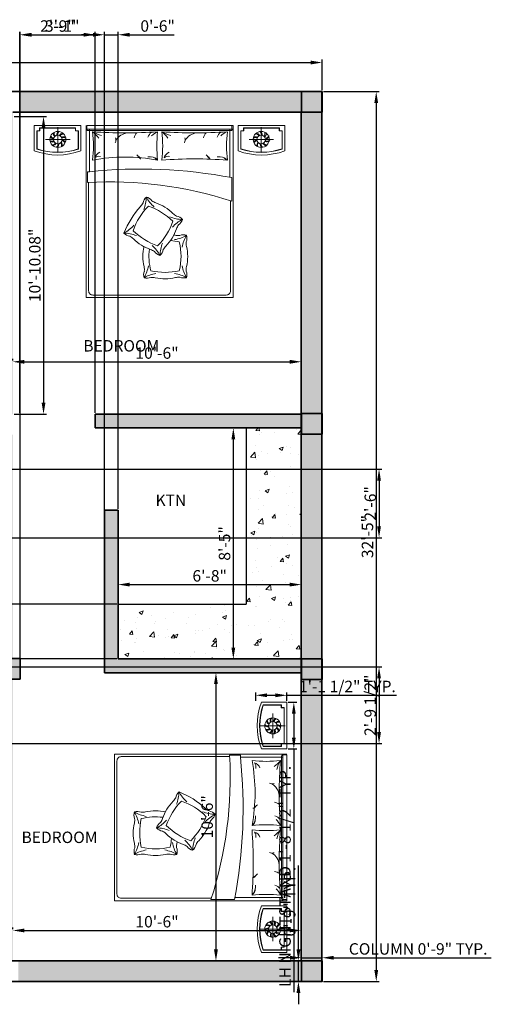
# Model space of a CAD drawing. Units: inches. Extents: x -36 to 490, y -420 to 94.
# Tile 4 of 4: x 284 to 490, y -385 to 45. Entities that reach past the tile are written whole.
import ezdxf

# ---------------------------------------------------------------- set-up
doc = ezdxf.new("R2010")
doc.units = ezdxf.units.IN
for name, color, linetype, lineweight in [('A-ANNO-DIMS', 2, 'Continuous', 18), ('A-AREA-IDEN', 1, 'Continuous', 18), ('A-COLS', 1, 'Continuous', 35), ('A-FLOR-FIXT', 8, 'Continuous', 25), ('A-FLOR-FIXT-PATT', 252, 'Continuous', 13), ('A-WALL', 7, 'Continuous', 35), ('furn', 8, 'Continuous', 18)]:
    doc.layers.add(name, color=color, linetype=linetype, lineweight=lineweight)
doc.layers.add('A-WALL-PATT', color=177, linetype='Continuous', lineweight=13, true_color=0x293189)
doc.styles.get("Standard").update_dxf_attribs({"font": 'arial.ttf'})
doc.dimstyles.new('ISO-25', dxfattribs={"dimtxt": 5, "dimasz": 5, "dimexe": 1.25, "dimexo": 0.625, "dimtad": 1, "dimlunit": 3, "dimtxsty": 'Standard', "dimcen": 2.5, "dimadec": 0, "dimazin": 0, "dimtfac": 1, "dimtmove": 0, "dimatfit": 3, "dimfxl": 1, "dimarcsym": 0})

# ---------------------------------------------------------------- blocks, each defined once
blk = doc.blocks.new('*D1')
at = {"layer": 'A-ANNO-DIMS', "color": 0, "lineweight": -2, "transparency": 16777216}
for p, q in [((280.98, -352.29), (280.98, -351.67)), ((285.98, -352.92), (401.98, -352.92)), ((406.98, -352.29), (406.98, -351.67))]:
    blk.add_line(p, q, dxfattribs=at)
at = {"layer": 'A-ANNO-DIMS', "color": 0, "transparency": 16777216}
for points in [[(285.98, -352.09), (285.98, -353.75), (280.98, -352.92)], [(401.98, -352.09), (401.98, -353.75), (406.98, -352.92)]]:
    blk.add_solid(points, dxfattribs=at)
at = {"layer": 'Defpoints', "color": 0, "transparency": 16777216}
for p in [(280.98, -352.92), (406.98, -352.92), (406.98, -352.92)]:
    blk.add_point(p, dxfattribs=at)
at = {"layer": 'A-ANNO-DIMS', "color": 0, "transparency": 16777216, "insert": (343.98, -349.74), "char_height": 5, "attachment_point": 5}
blk.add_mtext('10\'-6"', dxfattribs=at)
blk = doc.blocks.new('*D2')
at = {"layer": 'A-ANNO-DIMS', "color": 0, "lineweight": -2, "transparency": 16777216}
for p, q in [((347.38, -240.23), (370.97, -240.23)), ((369.72, -245.23), (369.72, -361.23)), ((347.38, -366.23), (370.97, -366.23))]:
    blk.add_line(p, q, dxfattribs=at)
at = {"layer": 'A-ANNO-DIMS', "color": 0, "transparency": 16777216}
for points in [[(368.88, -245.23), (370.55, -245.23), (369.72, -240.23)], [(368.88, -361.23), (370.55, -361.23), (369.72, -366.23)]]:
    blk.add_solid(points, dxfattribs=at)
at = {"layer": 'Defpoints', "color": 0, "transparency": 16777216}
for p in [(346.75, -240.23), (346.75, -366.23), (369.72, -366.23)]:
    blk.add_point(p, dxfattribs=at)
at = {"layer": 'A-ANNO-DIMS', "color": 0, "transparency": 16777216, "insert": (366.54, -303.23), "char_height": 5, "attachment_point": 5, "rotation": 90}
blk.add_mtext('10\'-6"', dxfattribs=at)
blk = doc.blocks.new('*D15')
at = {"layer": 'A-ANNO-DIMS', "color": 0, "lineweight": -2, "transparency": 16777216}
for p, q in [((281.61, 2.85), (295.66, 2.85)), ((294.41, -2.15), (294.41, -122.23)), ((281.61, -127.23), (295.66, -127.23))]:
    blk.add_line(p, q, dxfattribs=at)
at = {"layer": 'A-ANNO-DIMS', "color": 0, "transparency": 16777216}
for points in [[(293.58, -2.15), (295.25, -2.15), (294.41, 2.85)], [(293.58, -122.23), (295.25, -122.23), (294.41, -127.23)]]:
    blk.add_solid(points, dxfattribs=at)
at = {"layer": 'Defpoints', "color": 0, "transparency": 16777216}
for p in [(280.98, 2.85), (280.98, -127.23), (294.41, -127.23)]:
    blk.add_point(p, dxfattribs=at)
at = {"layer": 'A-ANNO-DIMS', "color": 0, "transparency": 16777216, "insert": (291.24, -62.19), "char_height": 5, "attachment_point": 5, "rotation": 90}
blk.add_mtext('10\'-10.08"', dxfattribs=at)
blk = doc.blocks.new('*D16')
at = {"layer": 'A-ANNO-DIMS', "color": 0, "lineweight": -2, "transparency": 16777216}
for p, q in [((280.98, -103.71), (280.98, -103.08)), ((406.98, -103.71), (406.98, -103.08)), ((285.98, -104.33), (401.98, -104.33))]:
    blk.add_line(p, q, dxfattribs=at)
at = {"layer": 'A-ANNO-DIMS', "color": 0, "transparency": 16777216}
for points in [[(285.98, -103.5), (285.98, -105.17), (280.98, -104.33)], [(401.98, -103.5), (401.98, -105.17), (406.98, -104.33)]]:
    blk.add_solid(points, dxfattribs=at)
at = {"layer": 'Defpoints', "color": 0, "transparency": 16777216}
for p in [(280.98, -104.33), (406.98, -104.33), (406.98, -104.33)]:
    blk.add_point(p, dxfattribs=at)
at = {"layer": 'A-ANNO-DIMS', "color": 0, "transparency": 16777216, "insert": (343.98, -101.16), "char_height": 5, "attachment_point": 5}
blk.add_mtext('10\'-6"', dxfattribs=at)
blk = doc.blocks.new('*D19')
at = {"layer": 'A-ANNO-DIMS', "color": 0, "lineweight": -2, "transparency": 16777216}
for p, q in [((326.98, -201.1), (326.98, -200.48)), ((331.98, -201.73), (401.98, -201.73)), ((406.98, -201.1), (406.98, -200.48))]:
    blk.add_line(p, q, dxfattribs=at)
at = {"layer": 'A-ANNO-DIMS', "color": 0, "transparency": 16777216}
for points in [[(331.98, -200.9), (331.98, -202.56), (326.98, -201.73)], [(401.98, -200.9), (401.98, -202.56), (406.98, -201.73)]]:
    blk.add_solid(points, dxfattribs=at)
at = {"layer": 'Defpoints', "color": 0, "transparency": 16777216}
for p in [(326.98, -201.73), (406.98, -201.73), (406.98, -201.73)]:
    blk.add_point(p, dxfattribs=at)
at = {"layer": 'A-ANNO-DIMS', "color": 0, "transparency": 16777216, "insert": (366.98, -198.55), "char_height": 5, "attachment_point": 5}
blk.add_mtext('6\'-8"', dxfattribs=at)
blk = doc.blocks.new('*D20')
at = {"layer": 'A-ANNO-DIMS', "color": 0, "lineweight": -2, "transparency": 16777216}
for p, q in [((366.67, -133.23), (378.56, -133.23)), ((377.31, -138.23), (377.31, -229.23)), ((366.67, -234.23), (378.56, -234.23))]:
    blk.add_line(p, q, dxfattribs=at)
at = {"layer": 'A-ANNO-DIMS', "color": 0, "transparency": 16777216}
for points in [[(376.48, -138.23), (378.14, -138.23), (377.31, -133.23)], [(376.48, -229.23), (378.14, -229.23), (377.31, -234.23)]]:
    blk.add_solid(points, dxfattribs=at)
at = {"layer": 'Defpoints', "color": 0, "transparency": 16777216}
for p in [(366.05, -133.23), (366.05, -234.23), (377.31, -234.23)]:
    blk.add_point(p, dxfattribs=at)
at = {"layer": 'A-ANNO-DIMS', "color": 0, "transparency": 16777216, "insert": (374.13, -183.73), "char_height": 5, "attachment_point": 5, "rotation": 90}
blk.add_mtext('8\'-5"', dxfattribs=at)
blk = doc.blocks.new('*D21')
at = {"layer": 'A-ANNO-DIMS', "color": 0, "lineweight": -2, "transparency": 16777216}
for p, q in [((-0.02, 14.4), (-0.02, 27.74)), ((4.98, 26.49), (411.1, 26.49)), ((416.1, 14.4), (416.1, 27.74))]:
    blk.add_line(p, q, dxfattribs=at)
at = {"layer": 'A-ANNO-DIMS', "color": 0, "transparency": 16777216}
for points in [[(4.98, 27.33), (4.98, 25.66), (-0.02, 26.49)], [(411.1, 27.33), (411.1, 25.66), (416.1, 26.49)]]:
    blk.add_solid(points, dxfattribs=at)
at = {"layer": 'Defpoints', "color": 0, "transparency": 16777216}
for p in [(416.1, 26.49), (-0.02, 13.77), (416.1, 13.77)]:
    blk.add_point(p, dxfattribs=at)
at = {"layer": 'A-ANNO-DIMS', "color": 0, "transparency": 16777216, "insert": (208.04, 29.67), "char_height": 5, "attachment_point": 5}
blk.add_mtext('34\'-8.11"', dxfattribs=at)
blk = doc.blocks.new('*D22')
at = {"layer": 'A-ANNO-DIMS', "color": 0, "lineweight": -2, "transparency": 16777216}
for p, q in [((416.72, 13.77), (440.97, 13.77)), ((439.72, 8.77), (439.72, -370.23)), ((416.72, -375.23), (440.97, -375.23))]:
    blk.add_line(p, q, dxfattribs=at)
at = {"layer": 'A-ANNO-DIMS', "color": 0, "transparency": 16777216}
for points in [[(438.89, 8.77), (440.55, 8.77), (439.72, 13.77)], [(438.89, -370.23), (440.55, -370.23), (439.72, -375.23)]]:
    blk.add_solid(points, dxfattribs=at)
at = {"layer": 'Defpoints', "color": 0, "transparency": 16777216}
for p in [(416.1, 13.77), (416.1, -375.23), (439.72, -375.23)]:
    blk.add_point(p, dxfattribs=at)
at = {"layer": 'A-ANNO-DIMS', "color": 0, "transparency": 16777216, "insert": (436.54, -180.73), "char_height": 5, "attachment_point": 5, "rotation": 90}
blk.add_mtext('32\'-5"', dxfattribs=at)
blk = doc.blocks.new('BED-DOUBLE')
for p, q in [((1.43, 73.57), (1.43, 55.04)), ((62.71, 73.57), (62.71, 52.63)), ((1.11, 73.01), (63.06, 73.01))]:
    blk.add_line(p, q)
for points in [[(0, 75.3), (0, 0), (64.18, 0), (64.18, 75.3)], [(63.58, 75.3), (63.58, 73.57), (0.37, 73.57), (0.37, 75.3), (64.18, 75.3)]]:
    blk.add_lwpolyline(points)
for points in [[(2.84, 60.1, 0.058596), (2.84, 72.5, 0.036889), (31.25, 72.5, 0.052163), (31.25, 60.1, 0.093111)], [(33.1, 60.1, 0.058596), (33.1, 72.5, 0.036648), (61.69, 72.5, 0.052163), (61.69, 60.1, 0.036967)], [(0.56, 55.04), (1.43, 55.04, -0.072944), (63.58, 52.45), (63.58, 42.16, 0.092568), (0.56, 50.32)]]:
    blk.add_lwpolyline(points, format="xyb", close=True)
for points in [[(1.11, 50.35), (1.11, 2.97, 0.414214), (2.97, 1.11), (61.21, 1.11, 0.414214), (63.06, 2.97), (63.06, 42.34)], [(25.2, 38.53, 0.091296), (26.33, 43.97, 0.091296), (29.75, 39.6, 0.091296)], [(20.61, 29.25, 0.111006), (31.2, 22.66, 0.119549), (37.88, 33.38, 0.107813), (27.32, 40)], [(27.26, 39.98, 0.121865), (20.61, 29.25, 0.121865)], [(36.64, 35.3, 0.091296), (42.07, 34.16, 0.091296), (37.69, 30.75, 0.091296)], [(21.95, 27.08, 0.091296), (16.52, 28.23, 0.091296), (20.9, 31.63, 0.091296)], [(32.26, 18.42, 0.159461), (33.7, 20.96, -0.076283), (34.84, 22.55, 0.115075), (39.49, 30.02, -0.076283), (40.42, 31.75, 0.159461), (42.07, 34.16)], [(38.64, 25.34, 0.091296), (43.86, 27.24, 0.091296), (41.94, 22.03, 0.091296)], [(43.86, 8.69, 0.159461), (43.73, 11.61, -0.076283), (43.86, 13.56, 0.115075), (43.86, 22.37, -0.076283), (43.73, 24.32, 0.159461), (43.86, 27.24)], [(28.24, 11.72, 0.111006), (40.71, 11.73, 0.119549), (40.71, 24.36, 0.033212), (36.88, 24.95)], [(33.39, 23.85, 0.091296), (32.26, 18.42, 0.091296), (28.84, 22.79)], [(30.52, 10.59, 0.091296), (25.31, 8.69, 0.091296), (27.23, 13.9, 0.091296)], [(41.94, 13.9, 0.091296), (43.86, 8.69, 0.091296), (38.64, 10.59)]]:
    blk.add_lwpolyline(points, format="xyb")
for centre, radius, start, end in [((1.11, 74.12), 1.11, 180, 270), ((63.06, 74.12), 1.11, 270, 0), ((9.44, 82.87), 12.28, 237.5379, 257.5233), ((-6.45, 60.91), 14.86, 36.4935, 51.2792), ((9.94, 68.98), 3.08, 335.8927, 16.1192), ((18.86, 65.15), 6.88, 96.6849, 148.3182), ((25.81, 69.06), 4.82, 141.8174, 169.8987), ((31.91, 68.38), 5.19, 130.5354, 160.3558), ((35.15, 64), 9.35, 114.6457, 134.1585), ((23.8, 60.91), 14.86, 36.4935, 51.2792), ((39.69, 82.87), 12.28, 237.5379, 257.5233), ((40.19, 68.98), 3.08, 335.8927, 16.1192), ((49.11, 65.15), 6.88, 96.6849, 148.3182), ((56.06, 69.06), 4.82, 141.8174, 169.8987), ((62.16, 68.38), 5.19, 130.5354, 160.3558), ((65.4, 64), 9.35, 114.6457, 134.1585), ((7.73, 59.82), 4.12, 114.2916, 160.9896), ((5.59, 58.96), 2.82, 76.4823, 128.5563), ((11.2, 51.48), 15.49, 36.2085, 45.0849), ((22.66, 60.63), 1.04, 353.7543, 77.2187), ((27.63, 56.56), 5.07, 44.406, 96.8342), ((28.58, 58.33), 3.21, 33.6349, 90.8456), ((37.98, 59.82), 4.12, 114.2916, 160.9896), ((35.84, 58.96), 2.82, 76.4823, 128.5563), ((41.46, 51.48), 15.49, 36.2085, 45.0849), ((52.91, 60.63), 1.04, 353.7543, 77.2187), ((57.88, 56.56), 5.07, 44.406, 96.8342), ((58.83, 58.33), 3.21, 33.6349, 90.8456), ((29.5, 40.5), 4.7, 132.4658, 168.7065), ((25.09, 39.6), 4.54, 37.2937, 74.0973), ((54.12, 12.85), 40.62, 138.3818, 157.7644), ((19.15, 44.34), 6.44, 315.5854, 333.0343), ((32.54, 47.52), 6.44, 233.2983, 250.7472), ((24.23, 23.07), 19.38, 45.1307, 71.3884), ((42.4, 41.42), 6.44, 225.7718, 243.2208), ((38.72, 31.4), 4.34, 39.4726, 79.6505), ((19.98, 31.41), 4.7, 222.6522, 258.8929), ((16.17, 21.05), 6.44, 45.7718, 63.2208), ((34.58, 8.4), 19.38, 77.0576, 78.7033), ((40.3, 33.58), 6.44, 257.6988, 275.1477), ((42.47, 23.13), 4.34, 71.3996, 111.5774), ((34.34, 39.4), 19.38, 225.1307, 251.3884), ((44.18, 17.97), 19.38, 166.8711, 193.1289), ((53.75, 18.1), 26.29, 173.1956, 194.0284), ((26.03, 14.95), 6.44, 53.2983, 70.7472), ((34.07, 23.48), 5.38, 218.7754, 250.3571), ((19.02, 12.17), 6.44, 355.0387, 12.4877), ((29.84, 9.96), 4.7, 159.3666, 195.6073), ((26.56, 13.23), 4.7, 254.5791, 290.8198), ((28.81, 2.42), 6.44, 77.6988, 95.1477), ((34.52, 27.6), 19.38, 257.0576, 283.3153), ((40.4, 2.45), 6.44, 85.2252, 102.6741), ((42.71, 13.95), 5.38, 250.7023, 282.284)]:
    blk.add_arc(centre, radius, start, end)
blk = doc.blocks.new('NIGHTSTAND-LAMP-L')
for p, q in [((10.31, 1.49), (10.31, 12.19)), ((4.96, 6.84), (15.66, 6.84))]:
    blk.add_line(p, q)
blk.add_lwpolyline([(0, 1.86), (0, 12.98), (20.4, 12.98), (20.4, 1.86, -0.181818)], format="xyb", close=True)
for points in [[(2.34, 11.87), (2.34, 10.65), (1.11, 10.65)], [(2.45, 11.87), (2.45, 10.54), (1.11, 10.54)], [(2.34, 11.87), (18.07, 11.87)], [(2.34, 11.76), (18.07, 11.76)], [(17.95, 11.87), (17.95, 10.54), (19.29, 10.54)], [(18.07, 11.87), (18.07, 10.65), (19.29, 10.65)]]:
    blk.add_lwpolyline(points)
for points in [[(19.29, 10.65), (19.29, 2.63, -0.167087), (1.11, 2.63), (1.11, 10.65)], [(19.18, 10.65), (19.18, 2.71, -0.165559), (1.22, 2.71), (1.22, 10.65)]]:
    blk.add_lwpolyline(points, format="xyb")
for radius in [3.49, 1.89]:
    blk.add_circle((10.31, 6.84), radius)
for centre, radius, start, end in [((10.62, 9.46), 2.24, 172.17, 218.4897), ((10.4, 9.41), 1.71, 160.3002, 220.538), ((12.1, 8.78), 2.24, 136.17, 182.4897), ((11.89, 8.87), 1.71, 124.3002, 184.538), ((12.89, 7.36), 2.24, 100.17, 146.4897), ((12.78, 7.55), 1.71, 88.3002, 148.538), ((7.89, 7.72), 1.71, 232.3002, 292.538), ((7.91, 7.94), 2.24, 244.17, 290.4897), ((9.02, 9.14), 2.24, 208.17, 254.4897), ((8.87, 8.97), 1.71, 196.3002, 256.538), ((7.84, 6.13), 1.71, 268.3002, 328.538), ((7.72, 6.33), 2.24, 280.17, 326.4897), ((8.72, 4.82), 1.71, 304.3002, 4.538), ((8.52, 4.9), 2.24, 316.17, 2.4897), ((10.22, 4.27), 1.71, 340.3002, 40.538), ((10, 4.22), 2.24, 352.17, 38.4897), ((12.7, 5.74), 2.24, 64.17, 110.4897), ((12.72, 5.96), 1.71, 52.3002, 112.538), ((11.74, 4.71), 1.71, 16.3002, 76.538), ((11.59, 4.54), 2.24, 28.17, 74.4897)]:
    blk.add_arc(centre, radius, start, end)
blk = doc.blocks.new('NIGHTSTAND-LAMP-R')
for p, q in [((10.1, 1.49), (10.1, 12.18)), ((15.45, 6.83), (4.75, 6.83))]:
    blk.add_line(p, q)
blk.add_lwpolyline([(20.4, 1.85), (20.4, 12.98), (0, 12.98), (0, 1.85, 0.181818)], format="xyb", close=True)
for points in [[(2.34, 11.87), (2.34, 10.65), (1.11, 10.65)], [(2.45, 11.87), (2.45, 10.53), (1.11, 10.53)], [(18.07, 11.87), (2.34, 11.87)], [(18.07, 11.76), (2.34, 11.76)], [(17.95, 11.87), (17.95, 10.53), (19.29, 10.53)], [(18.07, 11.87), (18.07, 10.65), (19.29, 10.65)]]:
    blk.add_lwpolyline(points)
for points in [[(1.11, 10.65), (1.11, 2.63, 0.167087), (19.29, 2.63), (19.29, 10.65)], [(1.22, 10.65), (1.22, 2.71, 0.165559), (19.18, 2.71), (19.18, 10.65)]]:
    blk.add_lwpolyline(points, format="xyb")
for radius in [3.49, 1.89]:
    blk.add_circle((10.1, 6.83), radius)
for centre, radius, start, end in [((7.62, 7.54), 1.71, 31.462, 91.6998), ((7.51, 7.35), 2.24, 33.5103, 79.83), ((8.51, 8.86), 1.71, 355.462, 55.6998), ((8.31, 8.77), 2.24, 357.5103, 43.83), ((10.01, 9.4), 1.71, 319.462, 19.6998), ((10.04, 9.55), 2.24, 321.5103, 7.83), ((7.68, 5.95), 1.71, 67.462, 127.6998), ((7.7, 5.73), 2.24, 69.5103, 115.83), ((8.81, 4.54), 2.24, 105.5103, 151.83), ((8.66, 4.7), 1.71, 103.462, 163.6998), ((10.41, 4.22), 2.24, 141.5103, 187.83), ((10.19, 4.27), 1.71, 139.462, 199.6998), ((11.88, 4.9), 2.24, 177.5103, 223.83), ((11.68, 4.81), 1.71, 175.462, 235.6998), ((12.68, 6.32), 2.24, 213.5103, 259.83), ((12.57, 6.13), 1.71, 211.462, 271.6998), ((12.74, 8.03), 2.24, 249.5103, 295.83), ((12.77, 7.81), 1.71, 247.462, 307.6998), ((11.79, 9.06), 1.71, 283.462, 343.6998), ((11.64, 9.23), 2.24, 285.5103, 331.83)]:
    blk.add_arc(centre, radius, start, end)
blk = doc.blocks.new('COLUMN-9X9')
h = blk.add_hatch(color=256)
h.dxf.hatch_style = 1
h.paths.add_polyline_path([(9, 0), (9, 9), (0, 9), (0, 0)])
blk.add_lwpolyline([(0, 9), (9, 9), (9, 0), (0, 0)], close=True)
blk = doc.blocks.new('*D28')
at = {"layer": 'A-ANNO-DIMS', "color": 0, "lineweight": -2, "transparency": 16777216}
for p, q in [((402.09, -364.85), (397.09, -364.85)), ((407.09, -365.57), (407.09, -363.6)), ((407.09, -364.85), (416.09, -364.85)), ((416.09, -365.57), (416.09, -363.6)), ((421.09, -364.85), (489.97, -364.85))]:
    blk.add_line(p, q, dxfattribs=at)
at = {"layer": 'A-ANNO-DIMS', "color": 0, "transparency": 16777216}
for points in [[(402.09, -364.01), (402.09, -365.68), (407.09, -364.85)], [(421.09, -364.01), (421.09, -365.68), (416.09, -364.85)]]:
    blk.add_solid(points, dxfattribs=at)
at = {"layer": 'Defpoints', "color": 0, "transparency": 16777216}
for p in [(416.09, -364.85), (407.09, -366.2), (416.09, -366.2)]:
    blk.add_point(p, dxfattribs=at)
at = {"layer": 'A-ANNO-DIMS', "color": 0, "transparency": 16777216, "insert": (458.03, -361.63), "char_height": 5, "attachment_point": 5}
blk.add_mtext('COLUMN 0\'-9" TYP.', dxfattribs=at)
blk = doc.blocks.new('*D29')
at = {"layer": 'A-ANNO-DIMS', "color": 0, "lineweight": -2, "transparency": 16777216}
for p, q in [((405.74, -361.2), (405.74, -324.47)), ((406.47, -366.2), (404.49, -366.2)), ((405.74, -375.2), (405.74, -366.2)), ((406.47, -375.2), (404.49, -375.2)), ((405.74, -380.2), (405.74, -385.2))]:
    blk.add_line(p, q, dxfattribs=at)
at = {"layer": 'A-ANNO-DIMS', "color": 0, "transparency": 16777216}
for points in [[(404.91, -361.2), (406.58, -361.2), (405.74, -366.2)], [(404.91, -380.2), (406.58, -380.2), (405.74, -375.2)]]:
    blk.add_solid(points, dxfattribs=at)
at = {"layer": 'Defpoints', "color": 0, "transparency": 16777216}
for p in [(405.74, -366.2), (407.09, -366.2), (407.09, -375.2)]:
    blk.add_point(p, dxfattribs=at)
at = {"layer": 'A-ANNO-DIMS', "color": 0, "transparency": 16777216, "insert": (402.57, -340.33), "char_height": 5, "attachment_point": 5, "rotation": 90}
blk.add_mtext('0\'-9" TYP.', dxfattribs=at)
blk = doc.blocks.new('*D32')
at = {"layer": 'A-ANNO-DIMS', "color": 0, "lineweight": -2, "transparency": 16777216}
for p, q in [((401.3, -253.17), (404.99, -253.17)), ((403.74, -258.17), (403.74, -268.58)), ((401.3, -273.58), (404.99, -273.58)), ((403.74, -273.58), (403.74, -379.94))]:
    blk.add_line(p, q, dxfattribs=at)
at = {"layer": 'A-ANNO-DIMS', "color": 0, "transparency": 16777216}
for points in [[(402.9, -258.17), (404.57, -258.17), (403.74, -253.17)], [(402.9, -268.58), (404.57, -268.58), (403.74, -273.58)]]:
    blk.add_solid(points, dxfattribs=at)
at = {"layer": 'Defpoints', "color": 0, "transparency": 16777216}
for p in [(400.68, -253.17), (400.68, -273.58), (403.74, -273.58)]:
    blk.add_point(p, dxfattribs=at)
at = {"layer": 'A-ANNO-DIMS', "color": 0, "transparency": 16777216, "insert": (400.53, -329.26), "char_height": 5, "attachment_point": 5, "rotation": 90}
blk.add_mtext('LH NIGHTSTAND 1\'-8 1/2" TYP.', dxfattribs=at)
blk = doc.blocks.new('*D33')
at = {"layer": 'A-ANNO-DIMS', "color": 0, "lineweight": -2, "transparency": 16777216}
for p, q in [((387.08, -252.55), (387.08, -248.86)), ((400.68, -252.55), (400.68, -248.86)), ((392.08, -250.11), (395.68, -250.11)), ((400.68, -250.11), (448.59, -250.11))]:
    blk.add_line(p, q, dxfattribs=at)
at = {"layer": 'A-ANNO-DIMS', "color": 0, "transparency": 16777216}
for points in [[(392.08, -249.28), (392.08, -250.95), (387.08, -250.11)], [(395.68, -249.28), (395.68, -250.95), (400.68, -250.11)]]:
    blk.add_solid(points, dxfattribs=at)
at = {"layer": 'Defpoints', "color": 0, "transparency": 16777216}
for p in [(387.08, -253.17), (400.68, -250.11), (400.68, -253.17)]:
    blk.add_point(p, dxfattribs=at)
at = {"layer": 'A-ANNO-DIMS', "color": 0, "transparency": 16777216, "insert": (427.13, -246.9), "char_height": 5, "attachment_point": 5}
blk.add_mtext('1\'-1 1/2" TYP.', dxfattribs=at)
blk = doc.blocks.new('*D41')
at = {"layer": 'A-ANNO-DIMS', "color": 0, "lineweight": -2, "transparency": 16777216}
for p, q in [((326.36, -210.23), (-26.2, -210.23)), ((-24.95, -215.23), (-24.95, -229.23)), ((326.36, -234.23), (-26.2, -234.23))]:
    blk.add_line(p, q, dxfattribs=at)
at = {"layer": 'A-ANNO-DIMS', "color": 0, "transparency": 16777216}
for points in [[(-25.78, -215.23), (-24.12, -215.23), (-24.95, -210.23)], [(-25.78, -229.23), (-24.12, -229.23), (-24.95, -234.23)]]:
    blk.add_solid(points, dxfattribs=at)
at = {"layer": 'Defpoints', "color": 0, "transparency": 16777216}
for p in [(326.98, -210.23), (-24.95, -234.23), (326.98, -234.23)]:
    blk.add_point(p, dxfattribs=at)
at = {"layer": 'A-ANNO-DIMS', "color": 0, "transparency": 16777216, "insert": (-28.13, -222.23), "char_height": 5, "attachment_point": 5, "rotation": 90}
blk.add_mtext('2\'-0"', dxfattribs=at)
blk = doc.blocks.new('*D44')
at = {"layer": 'A-ANNO-DIMS', "color": 0, "lineweight": -2, "transparency": 16777216}
for p, q in [((284.01, -126.62), (284.01, 39.87)), ((316.98, -126.6), (316.98, 39.87)), ((289.01, 38.62), (311.98, 38.62))]:
    blk.add_line(p, q, dxfattribs=at)
at = {"layer": 'A-ANNO-DIMS', "color": 0, "transparency": 16777216}
for points in [[(289.01, 39.45), (289.01, 37.79), (284.01, 38.62)], [(311.98, 39.45), (311.98, 37.79), (316.98, 38.62)]]:
    blk.add_solid(points, dxfattribs=at)
at = {"layer": 'Defpoints', "color": 0, "transparency": 16777216}
for p in [(316.98, 38.62), (284.01, -127.24), (316.98, -127.23)]:
    blk.add_point(p, dxfattribs=at)
at = {"layer": 'A-ANNO-DIMS', "color": 0, "transparency": 16777216, "insert": (300.5, 41.8), "char_height": 5, "attachment_point": 5}
blk.add_mtext('2\'-9"', dxfattribs=at)
blk = doc.blocks.new('*D45')
at = {"layer": 'A-ANNO-DIMS', "color": 0, "lineweight": -2, "transparency": 16777216}
for p, q in [((95.61, -151.23), (442.2, -151.23)), ((440.95, -156.23), (440.95, -176.23)), ((101.61, -181.23), (442.2, -181.23))]:
    blk.add_line(p, q, dxfattribs=at)
at = {"layer": 'A-ANNO-DIMS', "color": 0, "transparency": 16777216}
for points in [[(440.11, -156.23), (441.78, -156.23), (440.95, -151.23)], [(440.11, -176.23), (441.78, -176.23), (440.95, -181.23)]]:
    blk.add_solid(points, dxfattribs=at)
at = {"layer": 'Defpoints', "color": 0, "transparency": 16777216}
for p in [(94.98, -151.23), (100.98, -181.23), (440.95, -181.23)]:
    blk.add_point(p, dxfattribs=at)
at = {"layer": 'A-ANNO-DIMS', "color": 0, "transparency": 16777216, "insert": (437.77, -166.23), "char_height": 5, "attachment_point": 5, "rotation": 90}
blk.add_mtext('2\'-6"', dxfattribs=at)
blk = doc.blocks.new('*D47')
at = {"layer": 'A-ANNO-DIMS', "color": 0, "lineweight": -2, "transparency": 16777216}
for p, q in [((144.42, -237.73), (442.2, -237.73)), ((440.95, -242.73), (440.95, -266.23)), ((141.61, -271.23), (442.2, -271.23))]:
    blk.add_line(p, q, dxfattribs=at)
at = {"layer": 'A-ANNO-DIMS', "color": 0, "transparency": 16777216}
for points in [[(440.11, -242.73), (441.78, -242.73), (440.95, -237.73)], [(440.11, -266.23), (441.78, -266.23), (440.95, -271.23)]]:
    blk.add_solid(points, dxfattribs=at)
at = {"layer": 'Defpoints', "color": 0, "transparency": 16777216}
for p in [(143.79, -237.73), (140.98, -271.23), (440.95, -271.23)]:
    blk.add_point(p, dxfattribs=at)
at = {"layer": 'A-ANNO-DIMS', "color": 0, "transparency": 16777216, "insert": (437.74, -254.48), "char_height": 5, "attachment_point": 5, "rotation": 90}
blk.add_mtext('2\'-9 1/2"', dxfattribs=at)
blk = doc.blocks.new('*D48')
at = {"layer": 'A-ANNO-DIMS', "color": 0, "lineweight": -2, "transparency": 16777216}
for p, q in [((284.18, -242.43), (284.18, 39.87)), ((320.98, -239.6), (320.98, 39.87)), ((289.18, 38.62), (315.98, 38.62))]:
    blk.add_line(p, q, dxfattribs=at)
at = {"layer": 'A-ANNO-DIMS', "color": 0, "transparency": 16777216}
for points in [[(289.18, 39.45), (289.18, 37.79), (284.18, 38.62)], [(315.98, 39.45), (315.98, 37.79), (320.98, 38.62)]]:
    blk.add_solid(points, dxfattribs=at)
at = {"layer": 'Defpoints', "color": 0, "transparency": 16777216}
for p in [(320.98, 38.62), (320.98, -240.23), (284.18, -243.05)]:
    blk.add_point(p, dxfattribs=at)
at = {"layer": 'A-ANNO-DIMS', "color": 0, "transparency": 16777216, "insert": (302.58, 41.8), "char_height": 5, "attachment_point": 5}
blk.add_mtext('3\'-1"', dxfattribs=at)
blk = doc.blocks.new('*D49')
at = {"layer": 'A-ANNO-DIMS', "color": 0, "lineweight": -2, "transparency": 16777216}
for p, q in [((320.98, -168.6), (320.98, 39.87)), ((326.98, -168.6), (326.98, 39.87)), ((315.98, 38.62), (310.98, 38.62)), ((320.98, 38.62), (326.98, 38.62)), ((331.98, 38.62), (351.53, 38.62))]:
    blk.add_line(p, q, dxfattribs=at)
at = {"layer": 'A-ANNO-DIMS', "color": 0, "transparency": 16777216}
for points in [[(315.98, 39.45), (315.98, 37.79), (320.98, 38.62)], [(331.98, 39.45), (331.98, 37.79), (326.98, 38.62)]]:
    blk.add_solid(points, dxfattribs=at)
at = {"layer": 'Defpoints', "color": 0, "transparency": 16777216}
for p in [(326.98, 38.62), (320.98, -169.23), (326.98, -169.23)]:
    blk.add_point(p, dxfattribs=at)
at = {"layer": 'A-ANNO-DIMS', "color": 0, "transparency": 16777216, "insert": (344.25, 41.8), "char_height": 5, "attachment_point": 5}
blk.add_mtext('0\'-6"', dxfattribs=at)

msp = doc.modelspace()

# ---------------------------------------------------------------- hatches: boundary and pattern name
at = {"layer": 'A-FLOR-FIXT-PATT'}
h = msp.add_hatch(dxfattribs=at)
h.set_pattern_fill('AR-CONC', color=256, scale=0.1)
h.set_pattern_definition([(50, (-137.025, -13.273), (18.21847, -1.5939), [1.905, -20.955]), (355, (-137.025, -13.273), (-3.52434, 19.1057), [1.524, -16.76406]), (100.4514, (-135.507, -13.406), (14.6941, 17.5118), [1.619, -17.809]), (46.184, (-137.025, -8.193), (27.1079, -4.2042), [2.8575, -31.4325]), (96.6356, (-134.766, -8.544), (23.7404, 24.7426), [2.4285, -26.7136]), (351.184, (-137.025, -8.193), (23.7404, 24.7426), [2.286, -25.146]), (21, (-134.485, -9.463), (15.16144, -10.22652), [1.905, -20.955]), (326, (-134.485, -9.463), (6.1802, 18.4188), [1.524, -16.764]), (71.4514, (-133.222, -10.316), (21.34164, 8.1923), [1.619, -17.809]), (37.5, (-137.025, -13.2735), (0.30886, 8.455504), [0, -16.5608, 0, -17.018, 0, -16.8275]), (7.5, (-137.025, -13.2735), (6.68197, 10.01806), [0, -9.7028, 0, -16.1798, 0, -6.4135]), (327.5, (-142.6895, -13.2735), (13.55906, -0.572874), [0, -6.35, 0, -19.812, 0, -26.289]), (317.5, (-145.23, -13.273), (14.81292, 2.54265), [0, -8.255, 0, -13.1572, 0, -18.669])])
h.paths.add_polyline_path([(406.984, -133.228), (382.984, -133.228), (382.984, -210.228), (326.984, -210.228), (326.984, -234.228), (406.984, -234.228)])
at = {"layer": 'A-WALL-PATT'}
h = msp.add_hatch(color=256, dxfattribs=at)
h.dxf.hatch_style = 1
h.paths.add_polyline_path([(132.114, 13.772), (8.901, 13.772), (8.901, 4.772), (132.114, 4.772)])
h.paths.add_polyline_path([(274.98, 13.772), (141.114, 13.772), (141.114, 4.772), (274.98, 4.772)])
h.paths.add_polyline_path([(407.097, 13.772), (283.98, 13.772), (283.98, 4.772), (407.097, 4.772)])
h.paths.add_polyline_path([(280.984, 4.772), (274.984, 4.772), (274.984, -127.228), (280.984, -127.228)])
h.paths.add_polyline_path([(274.984, -127.228), (176.984, -127.228), (176.984, -133.228), (274.984, -133.228)])
h.paths.add_polyline_path([(140.984, 4.772), (134.984, 4.772), (134.984, -128.829), (140.984, -128.829)])
h.paths.add_polyline_path([(8.984, 4.772), (8.901, 4.772), (-0.016, 4.772), (-0.016, -127.003), (8.984, -127.003)])
h.paths.add_polyline_path([(94.984, -127.228), (8.984, -127.228), (8.984, -133.228), (88.984, -133.228), (88.984, -151.228), (94.984, -151.228), (94.984, -133.228)])
h.paths.add_polyline_path([(8.984, -136.003), (-0.016, -136.003), (-0.016, -228.965), (8.984, -228.965)])
h.paths.add_polyline_path([(100.984, -181.228), (98.984, -181.228), (88.984, -181.228), (8.984, -181.228), (8.984, -187.228), (88.984, -187.228), (94.984, -187.228), (94.984, -235.228), (134.793, -235.228), (134.793, -229.228), (100.984, -229.228)])
h.paths.add_polyline_path([(64.984, -229.228), (9.003, -229.228), (9.003, -235.228), (64.984, -235.228)], flags=17)
h.paths.add_polyline_path([(8.984, -237.965), (-0.016, -237.965), (-0.016, -366.285), (8.984, -366.285)])
h.paths.add_polyline_path([(132.054, -366.228), (9.018, -366.228), (9.018, -375.228), (132.054, -375.228)])
h.paths.add_polyline_path([(140.984, -271.228), (134.984, -271.228), (134.984, -366.131), (140.984, -366.131)])
h = msp.add_hatch(color=256, dxfattribs=at)
h.dxf.hatch_style = 1
h.paths.add_polyline_path([(280.984, -136.244), (274.984, -136.244), (274.984, -234.05), (280.984, -234.05)])
h.paths.add_polyline_path([(406.984, -127.228), (316.984, -127.228), (316.984, -133.228), (406.984, -133.228)])
h.paths.add_polyline_path([(415.984, 4.772), (406.984, 4.772), (406.984, -126.964), (415.984, -126.964)])
h = msp.add_hatch(color=256, dxfattribs=at)
h.dxf.hatch_style = 1
h.paths.add_polyline_path([(326.984, -169.228), (320.984, -169.228), (320.984, -240.228), (406.984, -240.228), (406.984, -234.228), (326.984, -234.228)])
h.paths.add_polyline_path([(415.984, -135.964), (406.984, -135.964), (406.984, -234.15), (415.984, -234.15)])
h = msp.add_hatch(color=256, dxfattribs=at)
h.dxf.hatch_style = 1
h.paths.add_polyline_path([(407.094, -366.228), (283.341, -366.228), (283.341, -375.228), (407.094, -375.228)])
h.paths.add_polyline_path([(415.984, -243.15), (406.984, -243.15), (406.984, -366.196), (415.984, -366.196)])
h.paths.add_polyline_path([(280.984, -243.05), (274.984, -243.05), (274.984, -366.161), (280.984, -366.161)])
h.paths.add_polyline_path([(274.341, -366.228), (182.984, -366.228), (182.984, -375.228), (183.401, -375.228), (274.341, -375.228)])

# ---------------------------------------------------------------- linework, layer by layer
at = {"layer": 'A-FLOR-FIXT'}
for p in [(382.984, -133.228), (326.984, -210.228)]:
    msp.add_line(p, (382.984, -210.228), dxfattribs=at)
at = {"layer": 'A-WALL'}
for p, q in [((280.984, 4.772), (406.984, 4.772)), ((406.984, 4.772), (406.984, -366.228)), ((316.984, -127.228), (406.984, -127.228)), ((316.984, -127.228), (316.984, -133.228)), ((316.984, -133.228), (406.984, -133.228)), ((320.984, -240.228), (320.984, -169.228)), ((326.984, -169.228), (320.984, -169.228)), ((326.984, -234.228), (326.984, -169.228)), ((326.984, -234.228), (406.984, -234.228)), ((320.984, -240.228), (406.984, -240.228)), ((406.984, -366.228), (274.984, -366.228))]:
    msp.add_line(p, q, dxfattribs=at)
msp.add_lwpolyline([(-0.016, 13.772), (415.984, 13.772), (415.984, -375.228), (-0.016, -375.228)], close=True, dxfattribs=at)

# ---------------------------------------------------------------- block references
at = {"layer": 'A-COLS'}
for p, rotation in [((407.096, 13.772), 269.9999999999993), ((407.073, -126.964), 269.9999999999998), ((275.178, -234.05), 269.9999999999997), ((407.086, -234.15), 269.9999999999998)]:
    msp.add_blockref('COLUMN-9X9', p, dxfattribs=dict(at, rotation=rotation))
msp.add_blockref('COLUMN-9X9', (407.094, -375.196), dxfattribs=at)
at = {"layer": 'furn'}
for name, p in [('NIGHTSTAND-LAMP-L', (290.375, -13.963)), ('BED-DOUBLE', (313.003, -76.278)), ('NIGHTSTAND-LAMP-R', (379.404, -13.958))]:
    msp.add_blockref(name, p, dxfattribs=at)
for name, p, rotation in [('NIGHTSTAND-LAMP-L', (387.694, -253.173), 270.0000000000005), ('BED-DOUBLE', (325.379, -275.801), 270.0000000000002), ('NIGHTSTAND-LAMP-R', (387.699, -342.202), 270.0000000000012)]:
    msp.add_blockref(name, p, dxfattribs=dict(at, rotation=rotation))

# ---------------------------------------------------------------- texts
at = {"layer": 'A-AREA-IDEN', "char_height": 5, "attachment_point": 1}
for s, width, insert in [('{BEDROOM}', 53.6263, (311.776, -94.849)), ('{KTN}', 30.63342, (343.319, -162.383)), ('{BEDROOM}', 40.58337, (284.796, -309.7))]:
    msp.add_mtext_dynamic_manual_height_columns(s, width=width, gutter_width=12.5, heights=[0], dxfattribs=dict(at, insert=insert))

# ---------------------------------------------------------------- dimensions: what is measured, and where the dimension line sits
at = {"layer": 'A-ANNO-DIMS'}
for base, p1, p2, override, picture, middle in [((316.984, 38.622), (284.01, -127.244), (316.984, -127.228), {"dimdec": 1, "dimlfac": 1, "dimrnd": 0, "dimzin": 1, "dimdsep": 46, "dimlunit": 4, "dimfrac": 2}, '*D44', (300.497, 41.799)), ((320.984, 38.622), (284.178, -243.05), (320.984, -240.228), {"dimdec": 1, "dimlfac": 1, "dimrnd": 0, "dimzin": 1, "dimdsep": 46, "dimlunit": 4, "dimfrac": 2}, '*D48', (302.581, 41.801)), ((326.984, 38.622), (320.984, -169.228), (326.984, -169.228), {"dimdec": 1, "dimlfac": 1, "dimrnd": 0, "dimzin": 1, "dimdsep": 46, "dimlunit": 4, "dimfrac": 2}, '*D49', (344.255, 41.799)), ((416.097, 26.492), (-0.016, 13.772), (416.097, 13.772), {"dimclrd": 0, "dimclre": 0, "dimclrt": 0}, '*D21', (208.04, 29.671)), ((406.984, -104.334), (280.984, -104.334), (406.984, -104.334), {"dimclrd": 0, "dimclre": 0, "dimclrt": 0}, '*D16', (343.984, -101.156)), ((406.984, -201.728), (326.984, -201.728), (406.984, -201.728), {"dimclrd": 0, "dimclre": 0, "dimclrt": 0}, '*D19', (366.984, -198.551)), ((406.984, -352.92), (280.984, -352.92), (406.984, -352.92), {"dimclrd": 0, "dimclre": 0, "dimclrt": 0}, '*D1', (343.984, -349.742))]:
    dim = msp.add_linear_dim(base=base, p1=p1, p2=p2, dimstyle='ISO-25', override=override, dxfattribs=at)
    dim.commit()
    dim.dimension.update_dxf_attribs({"geometry": picture, "text_midpoint": middle})
for base, p1, p2, override, picture, middle in [((439.72, -375.228), (416.097, 13.772), (416.097, -375.228), {"dimclrd": 0, "dimclre": 0, "dimclrt": 0}, '*D22', (436.541, -180.728)), ((294.414, -127.228), (280.984, 2.849), (280.984, -127.228), {"dimclrd": 0, "dimclre": 0, "dimclrt": 0}, '*D15', (291.236, -62.19)), ((377.308, -234.228), (366.045, -133.228), (366.045, -234.228), {"dimclrd": 0, "dimclre": 0, "dimclrt": 0}, '*D20', (374.131, -183.728)), ((440.947, -181.228), (94.984, -151.228), (100.984, -181.228), {"dimdec": 1, "dimlfac": 1, "dimrnd": 0, "dimzin": 1, "dimdsep": 46, "dimlunit": 4, "dimfrac": 2}, '*D45', (437.769, -166.228)), ((-24.949, -234.228), (326.984, -210.228), (326.984, -234.228), {"dimdec": 1, "dimlfac": 1, "dimrnd": 0, "dimzin": 1, "dimdsep": 46, "dimlunit": 4, "dimfrac": 2}, '*D41', (-28.126, -222.228)), ((440.947, -271.228), (143.793, -237.727), (140.984, -271.228), {"dimdec": 1, "dimlfac": 1, "dimrnd": 0, "dimzin": 1, "dimdsep": 46, "dimlunit": 4, "dimfrac": 2}, '*D47', (437.737, -254.478)), ((369.716, -366.228), (346.75, -240.228), (346.75, -366.228), {"dimclrd": 0, "dimclre": 0, "dimclrt": 0}, '*D2', (366.538, -303.228))]:
    dim = msp.add_linear_dim(base=base, p1=p1, p2=p2, angle=90, dimstyle='ISO-25', override=override, dxfattribs=at)
    dim.commit()
    dim.dimension.update_dxf_attribs({"geometry": picture, "text_midpoint": middle})
for base, p1, p2, angle, text, picture, middle in [((400.678, -250.112), (387.076, -253.173), (400.678, -253.173), 0, '<> TYP.', '*D33', (427.131, -246.902)), ((403.738, -273.575), (400.678, -253.173), (400.678, -273.575), 270, 'LH NIGHTSTAND <> TYP.', '*D32', (400.528, -329.26)), ((405.744, -366.196), (407.094, -375.196), (407.094, -366.196), 90, '<> TYP.', '*D29', (402.566, -340.332))]:
    dim = msp.add_linear_dim(base=base, p1=p1, p2=p2, angle=angle, text=text, dimstyle='ISO-25', override={"dimdec": 1, "dimlfac": 1, "dimrnd": 0, "dimzin": 1, "dimdsep": 46, "dimlunit": 4, "dimfrac": 2}, dxfattribs=at)
    dim.commit()
    dim.dimension.update_dxf_attribs({"geometry": picture, "text_midpoint": middle})
dim = msp.add_linear_dim(base=(416.094, -364.846), p1=(407.094, -366.196), p2=(416.094, -366.196), text='COLUMN <> TYP.', dimstyle='ISO-25', override={"dimdec": 1, "dimlfac": 1, "dimrnd": 0, "dimzin": 1, "dimdsep": 46, "dimlunit": 4, "dimfrac": 2}, dxfattribs=at)
dim.commit()
dim.dimension.update_dxf_attribs({"geometry": '*D28', "text_midpoint": (458.034, -361.634)})

doc.saveas('drawing.dxf')
